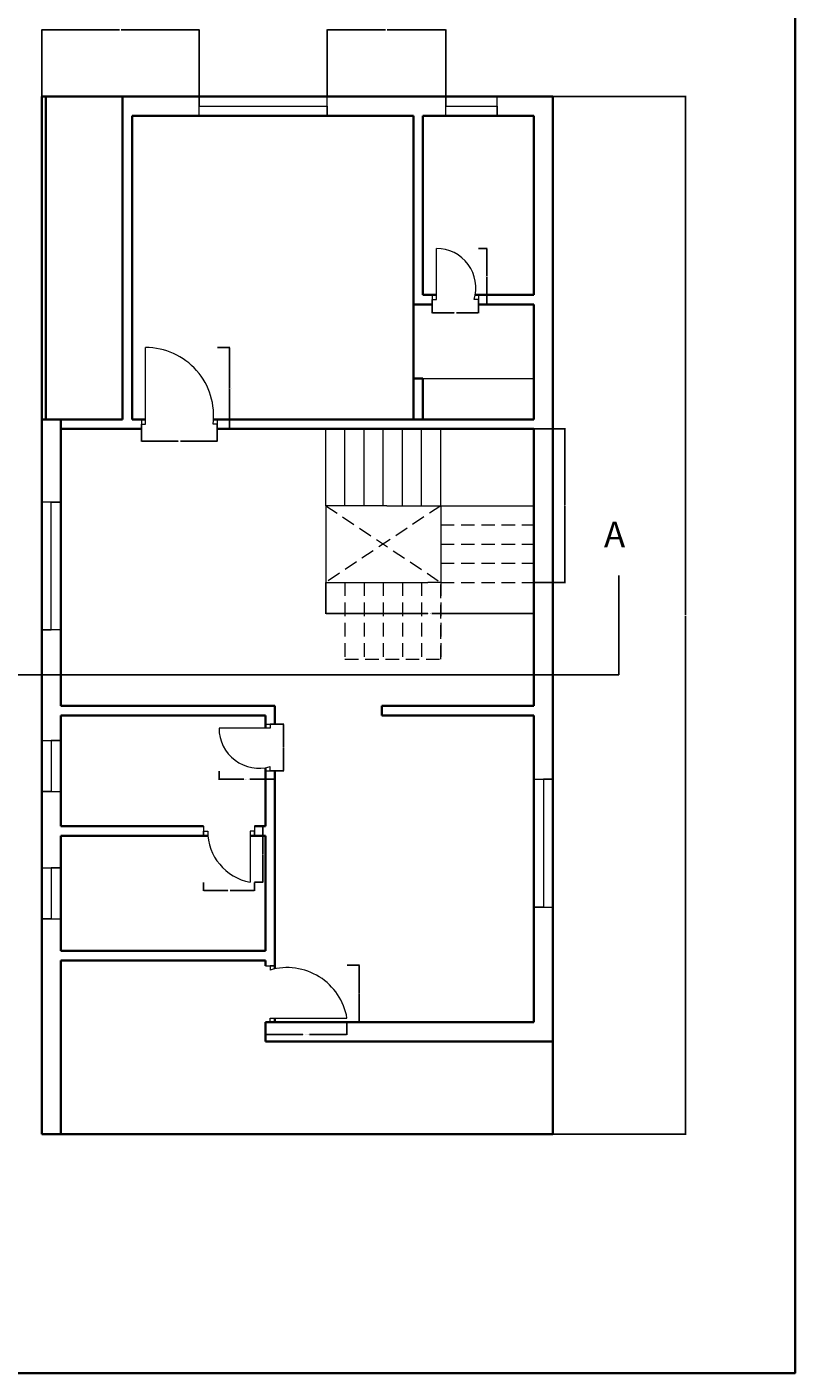
# Model space of a CAD drawing. Units: inches. Extents: x 1911 to 3278, y 2022 to 3108.
# Tile 12 of 13: x 2918 to 3278, y 2022 to 2654. Entities that reach past the tile are written whole.
import ezdxf

# ---------------------------------------------------------------- set-up
doc = ezdxf.new("R2010")
doc.units = ezdxf.units.IN
doc.linetypes.add('DASHED2', pattern=[9.525, 6.35, -3.175])
for name, color, linetype, lineweight in [('A-ANNO-DIMS', 2, 'Continuous', 18), ('A-ANNO-SYMB', 7, 'Continuous', 25), ('A-ANNO-TTLB', 7, 'Continuous', 35), ('A-DOOR', 4, 'Continuous', 18), ('A-FLOR-CASE', 9, 'Continuous', 18), ('A-FLOR-STRS', 7, 'Continuous', 18), ('A-FLOR-STRS-OVHD', 253, 'DASHED2', 13), ('A-GLAZ', 4, 'Continuous', 18), ('A-WALL', 7, 'Continuous', 35)]:
    doc.layers.add(name, color=color, linetype=linetype, lineweight=lineweight)
doc.styles.get("Standard").update_dxf_attribs({"font": 'arial.ttf'})
doc.dimstyles.get("Standard").update_dxf_attribs({"dimtxt": 0.18, "dimasz": 0.18, "dimexe": 0.18, "dimexo": 0.0625, "dimgap": 0.09, "dimtad": 0, "dimtih": 1, "dimtoh": 1, "dimdec": 4, "dimzin": 0, "dimdsep": 46, "dimtxsty": 'Standard', "dimcen": 0.09, "dimadec": 0, "dimazin": 0, "dimtfac": 1, "dimtdec": 4, "dimtofl": 0, "dimtmove": 0, "dimatfit": 3, "dimfxl": 1, "dimtolj": 1, "dimtzin": 0, "dimarcsym": 0})

# ---------------------------------------------------------------- blocks, each defined once
blk = doc.blocks.new('WIN-60')
for p, q in [((0, 60), (9, 60)), ((9, 60), (4.5, 60)), ((4.5, 60), (4.5, 0)), ((4.5, 0), (0, 0)), ((0, 0), (9, 0))]:
    blk.add_line(p, q)
blk = doc.blocks.new('WIN-24')
for p, q in [((0, 24), (9, 24)), ((9, 24), (4.5, 24)), ((4.5, 24), (4.5, 0)), ((4.5, 0), (0, 0)), ((0, 0), (9, 0))]:
    blk.add_line(p, q)
blk = doc.blocks.new('DOOR-BED-FF')
for p, q in [((2, 2.25), (2, 38.25)), ((0, 4.5), (0, 0)), ((0, 0), (0, 2.25)), ((0, 2.25), (2, 2.25)), ((35.66, 2.25), (33.66, 2.25)), ((35.66, 4.5), (35.66, 0)), ((35.66, 0), (35.66, 2.25))]:
    blk.add_line(p, q)
blk.add_arc((2, 6.33), 31.92, 352.65052, 90)
blk = doc.blocks.new('DOOR-BATH-FF')
for p, q in [((2, 2.25), (2, 26.25)), ((0, 4.5), (0, 0)), ((0, 0), (0, 2.25)), ((0, 2.25), (2, 2.25)), ((21.7, 2.25), (19.7, 2.25)), ((21.7, 4.5), (21.7, 0)), ((21.7, 0), (21.7, 2.25))]:
    blk.add_line(p, q)
blk.add_arc((2, 7.72), 18.53, 342.82983, 90)
blk = doc.blocks.new('DOOR-BALCONY')
for p, q in [((0, 26.53), (4.5, 26.53)), ((4.5, 26.53), (2.25, 26.53)), ((2.25, 26.53), (2.25, 24.53)), ((2.32, 0), (2.32, 2)), ((2.32, 2), (38.32, 2))]:
    blk.add_line(p, q)
blk.add_arc((10.23, -2.83), 28.5, 9.76334, 106.26632)
blk = doc.blocks.new('DOOR-DRESS-FF')
for p, q in [((24, 20), (0, 20)), ((21.75, 22), (26.25, 22)), ((26.25, 22), (24, 22)), ((24, 22), (24, 20)), ((21.75, 0), (26.25, 0)), ((24, 0), (24, 2)), ((26.25, 0), (24, 0))]:
    blk.add_line(p, q)
blk.add_arc((18.75, 20), 18.75, 180, 286.25091)
blk = doc.blocks.new('DOOR-ENSUITE-FF')
for p, q in [((0, 26.25), (0, 21.75)), ((23.93, 26.25), (23.93, 21.75)), ((0, 21.75), (0, 24)), ((0, 24), (0, 24)), ((0, 24), (2, 24)), ((23.93, 24), (21.93, 24)), ((21.93, 24), (21.93, 0)), ((23.93, 21.75), (23.93, 24))]:
    blk.add_line(p, q)
blk.add_arc((26.42, 24), 24.42, 180, 259.41225)
blk = doc.blocks.new('STAIR-PLAN-FF')
for p, q in [((0, 36), (0, 72)), ((9, 36), (9, 72)), ((18, 36), (18, 72)), ((27, 36), (27, 72)), ((36, 36), (36, 72)), ((45, 36), (45, 72)), ((54, 36), (54, 72)), ((28.63, 36), (0, 36)), ((0, 36), (0, 0)), ((28.63, 36), (97.65, 36)), ((54, 36), (54, 0)), ((54, 36), (54, 27)), ((0, 0), (48, 0)), ((54, 0), (48, 0))]:
    blk.add_line(p, q)
blk = doc.blocks.new('STAIR-BEYOND-FF')
for p, q in [((54, 72), (0, 36)), ((0, 72), (54, 36)), ((54, 72), (54, 63)), ((54, 63), (97.65, 63)), ((54, 54), (97.65, 54)), ((54, 45), (97.65, 45)), ((9, 36), (9, 0)), ((18, 36), (18, 0)), ((27, 36), (27, 0)), ((36, 36), (36, 0)), ((45, 36), (45, 0)), ((54, 36), (97.65, 36)), ((54, 0), (54, 36)), ((54, 36), (54, 0)), ((9, 0), (54, 0))]:
    blk.add_line(p, q)
blk = doc.blocks.new('*D46')
at = {"layer": 'A-ANNO-DIMS', "color": 0, "lineweight": -2, "transparency": 16777216}
for p, q in [((3007.14, 2503.12), (3012.99, 2503.12)), ((3012.81, 2502.94), (3012.81, 2484.18)), ((3012.81, 2465.05), (3012.81, 2483.82)), ((3007.14, 2464.87), (3012.99, 2464.87))]:
    blk.add_line(p, q, dxfattribs=at)
at = {"layer": 'A-ANNO-DIMS', "color": 0, "transparency": 16777216}
for points in [[(3012.78, 2502.94), (3012.84, 2502.94), (3012.81, 2503.12)], [(3012.78, 2465.05), (3012.84, 2465.05), (3012.81, 2464.87)]]:
    blk.add_solid(points, dxfattribs=at)
at = {"layer": 'Defpoints', "color": 0, "transparency": 16777216}
for p in [(3007.08, 2503.12), (3012.81, 2503.12), (3007.08, 2464.87)]:
    blk.add_point(p, dxfattribs=at)
at = {"layer": 'A-ANNO-DIMS', "color": 0, "transparency": 16777216, "insert": (3012.81, 2484), "char_height": 0.18, "attachment_point": 5}
blk.add_mtext('\\A1;BEDROOM DOOR 38 TYP.', dxfattribs=at)
blk = doc.blocks.new('*D47')
at = {"layer": 'A-ANNO-DIMS', "color": 0, "lineweight": -2, "transparency": 16777216}
for p, q in [((2971.42, 2464.81), (2971.42, 2458.96)), ((3007.08, 2464.81), (3007.08, 2458.96)), ((2971.6, 2459.14), (2988.72, 2459.14)), ((3006.9, 2459.14), (2989.78, 2459.14))]:
    blk.add_line(p, q, dxfattribs=at)
at = {"layer": 'A-ANNO-DIMS', "color": 0, "transparency": 16777216}
for points in [[(2971.6, 2459.17), (2971.6, 2459.11), (2971.42, 2459.14)], [(3006.9, 2459.17), (3006.9, 2459.11), (3007.08, 2459.14)]]:
    blk.add_solid(points, dxfattribs=at)
at = {"layer": 'Defpoints', "color": 0, "transparency": 16777216}
for p in [(2971.42, 2464.87), (3007.08, 2464.87), (3007.08, 2459.14)]:
    blk.add_point(p, dxfattribs=at)
at = {"layer": 'A-ANNO-DIMS', "color": 0, "transparency": 16777216, "insert": (2989.25, 2459.14), "char_height": 0.18, "attachment_point": 5}
blk.add_mtext('\\A1;36 TYP.', dxfattribs=at)
blk = doc.blocks.new('*D48')
at = {"layer": 'A-ANNO-DIMS', "color": 0, "lineweight": -2, "transparency": 16777216}
for p, q in [((3129.7, 2549.62), (3133.76, 2549.62)), ((3133.58, 2549.44), (3133.58, 2536.68)), ((3133.58, 2523.55), (3133.58, 2536.32)), ((3129.7, 2523.37), (3133.76, 2523.37))]:
    blk.add_line(p, q, dxfattribs=at)
at = {"layer": 'A-ANNO-DIMS', "color": 0, "transparency": 16777216}
for points in [[(3133.55, 2549.44), (3133.61, 2549.44), (3133.58, 2549.62)], [(3133.55, 2523.55), (3133.61, 2523.55), (3133.58, 2523.37)]]:
    blk.add_solid(points, dxfattribs=at)
at = {"layer": 'Defpoints', "color": 0, "transparency": 16777216}
for p in [(3129.64, 2549.62), (3133.58, 2549.62), (3129.64, 2523.37)]:
    blk.add_point(p, dxfattribs=at)
at = {"layer": 'A-ANNO-DIMS', "color": 0, "transparency": 16777216, "insert": (3133.58, 2536.5), "char_height": 0.18, "attachment_point": 5}
blk.add_mtext('\\A1;BATH DOOR 26 TYP.', dxfattribs=at)
blk = doc.blocks.new('*D49')
at = {"layer": 'A-ANNO-DIMS', "color": 0, "lineweight": -2, "transparency": 16777216}
for p, q in [((3107.93, 2523.31), (3107.93, 2519.26)), ((3129.64, 2523.31), (3129.64, 2519.26)), ((3108.11, 2519.44), (3118.26, 2519.44)), ((3129.46, 2519.44), (3119.32, 2519.44))]:
    blk.add_line(p, q, dxfattribs=at)
at = {"layer": 'A-ANNO-DIMS', "color": 0, "transparency": 16777216}
for points in [[(3108.11, 2519.47), (3108.11, 2519.41), (3107.93, 2519.44)], [(3129.46, 2519.47), (3129.46, 2519.41), (3129.64, 2519.44)]]:
    blk.add_solid(points, dxfattribs=at)
at = {"layer": 'Defpoints', "color": 0, "transparency": 16777216}
for p in [(3107.93, 2523.37), (3129.64, 2523.37), (3129.64, 2519.44)]:
    blk.add_point(p, dxfattribs=at)
at = {"layer": 'A-ANNO-DIMS', "color": 0, "transparency": 16777216, "insert": (3118.79, 2519.44), "char_height": 0.18, "attachment_point": 5}
blk.add_mtext('\\A1;22 TYP.', dxfattribs=at)
blk = doc.blocks.new('*D50')
at = {"layer": 'A-ANNO-DIMS', "color": 0, "lineweight": -2, "transparency": 16777216}
for p, q in [((3029.64, 2186.31), (3029.64, 2180.45)), ((3067.96, 2186.31), (3067.96, 2180.45)), ((3029.82, 2180.63), (3047.23, 2180.63)), ((3067.78, 2180.63), (3050.37, 2180.63))]:
    blk.add_line(p, q, dxfattribs=at)
at = {"layer": 'A-ANNO-DIMS', "color": 0, "transparency": 16777216}
for points in [[(3029.82, 2180.66), (3029.82, 2180.6), (3029.64, 2180.63)], [(3067.78, 2180.66), (3067.78, 2180.6), (3067.96, 2180.63)]]:
    blk.add_solid(points, dxfattribs=at)
at = {"layer": 'Defpoints', "color": 0, "transparency": 16777216}
for p in [(3029.64, 2186.37), (3067.96, 2186.37), (3067.96, 2180.63)]:
    blk.add_point(p, dxfattribs=at)
at = {"layer": 'A-ANNO-DIMS', "color": 0, "transparency": 16777216, "insert": (3048.8, 2180.63), "char_height": 0.18, "attachment_point": 5}
blk.add_mtext('\\A1;BALCONY DOOR 38 TYP.', dxfattribs=at)
blk = doc.blocks.new('*D51')
at = {"layer": 'A-ANNO-DIMS', "color": 0, "lineweight": -2, "transparency": 16777216}
for p, q in [((3068.02, 2213.17), (3073.89, 2213.17)), ((3073.71, 2212.99), (3073.71, 2199.95)), ((3073.71, 2186.55), (3073.71, 2199.59)), ((3068.02, 2186.37), (3073.89, 2186.37))]:
    blk.add_line(p, q, dxfattribs=at)
at = {"layer": 'A-ANNO-DIMS', "color": 0, "transparency": 16777216}
for points in [[(3073.68, 2212.99), (3073.74, 2212.99), (3073.71, 2213.17)], [(3073.68, 2186.55), (3073.74, 2186.55), (3073.71, 2186.37)]]:
    blk.add_solid(points, dxfattribs=at)
at = {"layer": 'Defpoints', "color": 0, "transparency": 16777216}
for p in [(3067.96, 2213.17), (3073.71, 2213.17), (3067.96, 2186.37)]:
    blk.add_point(p, dxfattribs=at)
at = {"layer": 'A-ANNO-DIMS', "color": 0, "transparency": 16777216, "insert": (3073.71, 2199.77), "char_height": 0.18, "attachment_point": 5}
blk.add_mtext('\\A1;27 TYP.', dxfattribs=at)
blk = doc.blocks.new('*D52')
at = {"layer": 'A-ANNO-DIMS', "color": 0, "lineweight": -2, "transparency": 16777216}
for p, q in [((3007.89, 2304.31), (3007.89, 2300.26)), ((3008.07, 2300.44), (3019.61, 2300.44)), ((3033.96, 2300.44), (3022.42, 2300.44)), ((3034.14, 2304.31), (3034.14, 2300.26))]:
    blk.add_line(p, q, dxfattribs=at)
at = {"layer": 'A-ANNO-DIMS', "color": 0, "transparency": 16777216}
for points in [[(3008.07, 2300.47), (3008.07, 2300.41), (3007.89, 2300.44)], [(3033.96, 2300.47), (3033.96, 2300.41), (3034.14, 2300.44)]]:
    blk.add_solid(points, dxfattribs=at)
at = {"layer": 'Defpoints', "color": 0, "transparency": 16777216}
for p in [(3007.89, 2304.37), (3034.14, 2304.37), (3034.14, 2300.44)]:
    blk.add_point(p, dxfattribs=at)
at = {"layer": 'A-ANNO-DIMS', "color": 0, "transparency": 16777216, "insert": (3021.01, 2300.44), "char_height": 0.18, "attachment_point": 5}
blk.add_mtext('\\A1;DRESS DOOR 26 TYP.', dxfattribs=at)
blk = doc.blocks.new('*D53')
at = {"layer": 'A-ANNO-DIMS', "color": 0, "lineweight": -2, "transparency": 16777216}
for p, q in [((3034.2, 2326.38), (3038.26, 2326.38)), ((3038.08, 2326.2), (3038.08, 2315.56)), ((3038.08, 2304.55), (3038.08, 2315.19)), ((3034.2, 2304.37), (3038.26, 2304.37))]:
    blk.add_line(p, q, dxfattribs=at)
at = {"layer": 'A-ANNO-DIMS', "color": 0, "transparency": 16777216}
for points in [[(3038.05, 2326.2), (3038.11, 2326.2), (3038.08, 2326.38)], [(3038.05, 2304.55), (3038.11, 2304.55), (3038.08, 2304.37)]]:
    blk.add_solid(points, dxfattribs=at)
at = {"layer": 'Defpoints', "color": 0, "transparency": 16777216}
for p in [(3034.14, 2326.38), (3038.08, 2326.38), (3034.14, 2304.37)]:
    blk.add_point(p, dxfattribs=at)
at = {"layer": 'A-ANNO-DIMS', "color": 0, "transparency": 16777216, "insert": (3038.08, 2315.37), "char_height": 0.18, "attachment_point": 5}
blk.add_mtext('\\A1;22 TYP.', dxfattribs=at)
blk = doc.blocks.new('*D54')
at = {"layer": 'A-ANNO-DIMS', "color": 0, "lineweight": -2, "transparency": 16777216}
for p, q in [((3024.55, 2278.37), (3028.61, 2278.37)), ((3028.43, 2278.19), (3028.43, 2265.43)), ((3028.43, 2252.3), (3028.43, 2265.07)), ((3024.55, 2252.12), (3028.61, 2252.12))]:
    blk.add_line(p, q, dxfattribs=at)
at = {"layer": 'A-ANNO-DIMS', "color": 0, "transparency": 16777216}
for points in [[(3028.4, 2278.19), (3028.46, 2278.19), (3028.43, 2278.37)], [(3028.4, 2252.3), (3028.46, 2252.3), (3028.43, 2252.12)]]:
    blk.add_solid(points, dxfattribs=at)
at = {"layer": 'Defpoints', "color": 0, "transparency": 16777216}
for p in [(3024.49, 2278.37), (3028.43, 2278.37), (3024.49, 2252.12)]:
    blk.add_point(p, dxfattribs=at)
at = {"layer": 'A-ANNO-DIMS', "color": 0, "transparency": 16777216, "insert": (3028.43, 2265.25), "char_height": 0.18, "attachment_point": 5}
blk.add_mtext('\\A1;ENSUITE DOOR 26 TYP.', dxfattribs=at)
blk = doc.blocks.new('*D55')
at = {"layer": 'A-ANNO-DIMS', "color": 0, "lineweight": -2, "transparency": 16777216}
for p, q in [((3000.56, 2252.06), (3000.56, 2248.01)), ((3024.49, 2252.06), (3024.49, 2248.01)), ((3000.74, 2248.19), (3011.99, 2248.19)), ((3024.31, 2248.19), (3013.05, 2248.19))]:
    blk.add_line(p, q, dxfattribs=at)
at = {"layer": 'A-ANNO-DIMS', "color": 0, "transparency": 16777216}
for points in [[(3000.74, 2248.22), (3000.74, 2248.16), (3000.56, 2248.19)], [(3024.31, 2248.22), (3024.31, 2248.16), (3024.49, 2248.19)]]:
    blk.add_solid(points, dxfattribs=at)
at = {"layer": 'Defpoints', "color": 0, "transparency": 16777216}
for p in [(3000.56, 2252.12), (3024.49, 2252.12), (3024.49, 2248.19)]:
    blk.add_point(p, dxfattribs=at)
at = {"layer": 'A-ANNO-DIMS', "color": 0, "transparency": 16777216, "insert": (3012.52, 2248.19), "char_height": 0.18, "attachment_point": 5}
blk.add_mtext('\\A1;24 TYP.', dxfattribs=at)
blk = doc.blocks.new('*D62')
at = {"layer": 'A-ANNO-DIMS', "color": 0, "lineweight": -2, "transparency": 16777216}
for p, q in [((3057.99, 2392.81), (3057.99, 2378.05)), ((3155.64, 2392.81), (3155.64, 2378.05)), ((3058.17, 2378.23), (3105.88, 2378.23)), ((3155.46, 2378.23), (3107.75, 2378.23))]:
    blk.add_line(p, q, dxfattribs=at)
at = {"layer": 'A-ANNO-DIMS', "color": 0, "transparency": 16777216}
for points in [[(3058.17, 2378.26), (3058.17, 2378.2), (3057.99, 2378.23)], [(3155.46, 2378.26), (3155.46, 2378.2), (3155.64, 2378.23)]]:
    blk.add_solid(points, dxfattribs=at)
at = {"layer": 'Defpoints', "color": 0, "transparency": 16777216}
for p in [(3057.99, 2392.87), (3155.64, 2392.87), (3155.64, 2378.23)]:
    blk.add_point(p, dxfattribs=at)
at = {"layer": 'A-ANNO-DIMS', "color": 0, "transparency": 16777216, "insert": (3106.81, 2378.23), "char_height": 0.18, "attachment_point": 5}
blk.add_mtext('\\A1;STAIR 98 TYP.', dxfattribs=at)
blk = doc.blocks.new('*D63')
at = {"layer": 'A-ANNO-DIMS', "color": 0, "lineweight": -2, "transparency": 16777216}
for p, q in [((3155.7, 2464.87), (3170.47, 2464.87)), ((3170.29, 2464.69), (3170.29, 2429.05)), ((3170.29, 2393.05), (3170.29, 2428.69)), ((3155.7, 2392.87), (3170.47, 2392.87))]:
    blk.add_line(p, q, dxfattribs=at)
at = {"layer": 'A-ANNO-DIMS', "color": 0, "transparency": 16777216}
for points in [[(3170.26, 2464.69), (3170.32, 2464.69), (3170.29, 2464.87)], [(3170.26, 2393.05), (3170.32, 2393.05), (3170.29, 2392.87)]]:
    blk.add_solid(points, dxfattribs=at)
at = {"layer": 'Defpoints', "color": 0, "transparency": 16777216}
for p in [(3155.64, 2464.87), (3170.29, 2464.87), (3155.64, 2392.87)]:
    blk.add_point(p, dxfattribs=at)
at = {"layer": 'A-ANNO-DIMS', "color": 0, "transparency": 16777216, "insert": (3170.29, 2428.87), "char_height": 0.18, "attachment_point": 5}
blk.add_mtext('\\A1;72 TYP.', dxfattribs=at)
blk = doc.blocks.new('*D84')
at = {"layer": 'A-ANNO-DIMS', "color": 0, "lineweight": -2, "transparency": 16777216}
for p, q in [((2924.64, 2620.94), (2924.64, 2652.45)), ((2924.82, 2652.27), (2961.22, 2652.27)), ((2998.41, 2652.27), (2962.01, 2652.27)), ((2998.59, 2620.94), (2998.59, 2652.45))]:
    blk.add_line(p, q, dxfattribs=at)
at = {"layer": 'A-ANNO-DIMS', "color": 0, "transparency": 16777216}
for points in [[(2924.82, 2652.3), (2924.82, 2652.24), (2924.64, 2652.27)], [(2998.41, 2652.3), (2998.41, 2652.24), (2998.59, 2652.27)]]:
    blk.add_solid(points, dxfattribs=at)
at = {"layer": 'Defpoints', "color": 0, "transparency": 16777216}
for p in [(2998.59, 2652.27), (2924.64, 2620.87), (2998.59, 2620.87)]:
    blk.add_point(p, dxfattribs=at)
at = {"layer": 'A-ANNO-DIMS', "color": 0, "transparency": 16777216, "insert": (2961.61, 2652.27), "char_height": 0.18, "attachment_point": 5}
blk.add_mtext('\\A1;73.95', dxfattribs=at)
blk = doc.blocks.new('*D85')
at = {"layer": 'A-ANNO-DIMS', "color": 0, "lineweight": -2, "transparency": 16777216}
for p, q in [((3058.59, 2620.94), (3058.59, 2652.45)), ((3058.77, 2652.27), (3086.11, 2652.27)), ((3114.23, 2652.27), (3086.89, 2652.27)), ((3114.41, 2620.94), (3114.41, 2652.45))]:
    blk.add_line(p, q, dxfattribs=at)
at = {"layer": 'A-ANNO-DIMS', "color": 0, "transparency": 16777216}
for points in [[(3058.77, 2652.3), (3058.77, 2652.24), (3058.59, 2652.27)], [(3114.23, 2652.3), (3114.23, 2652.24), (3114.41, 2652.27)]]:
    blk.add_solid(points, dxfattribs=at)
at = {"layer": 'Defpoints', "color": 0, "transparency": 16777216}
for p in [(3114.41, 2652.27), (3058.59, 2620.87), (3114.41, 2620.87)]:
    blk.add_point(p, dxfattribs=at)
at = {"layer": 'A-ANNO-DIMS', "color": 0, "transparency": 16777216, "insert": (3086.5, 2652.27), "char_height": 0.18, "attachment_point": 5}
blk.add_mtext('\\A1;55.83', dxfattribs=at)
blk = doc.blocks.new('*D86')
at = {"layer": 'A-ANNO-DIMS', "color": 0, "lineweight": -2, "transparency": 16777216}
for p, q in [((3164.7, 2620.87), (3227.12, 2620.87)), ((3226.94, 2620.69), (3226.94, 2377.56)), ((3226.94, 2134.05), (3226.94, 2377.19)), ((3164.7, 2133.87), (3227.12, 2133.87))]:
    blk.add_line(p, q, dxfattribs=at)
at = {"layer": 'A-ANNO-DIMS', "color": 0, "transparency": 16777216}
for points in [[(3226.91, 2620.69), (3226.97, 2620.69), (3226.94, 2620.87)], [(3226.91, 2134.05), (3226.97, 2134.05), (3226.94, 2133.87)]]:
    blk.add_solid(points, dxfattribs=at)
at = {"layer": 'Defpoints', "color": 0, "transparency": 16777216}
for p in [(3164.64, 2620.87), (3226.94, 2620.87), (3164.64, 2133.87)]:
    blk.add_point(p, dxfattribs=at)
at = {"layer": 'A-ANNO-DIMS', "color": 0, "transparency": 16777216, "insert": (3226.94, 2377.37), "char_height": 0.18, "attachment_point": 5}
blk.add_mtext('\\A1;487', dxfattribs=at)

msp = doc.modelspace()

# ---------------------------------------------------------------- linework, layer by layer
at = {"layer": 'A-ANNO-SYMB'}
for q in [(3195.5436, 2396.0454), (2593.3449, 2349.5267)]:
    msp.add_line((3195.5436, 2349.5267), q, dxfattribs=at)
at = {"layer": 'A-ANNO-TTLB'}
msp.add_lwpolyline([(1911.3875, 3108.0628), (3278.3142, 3108.0628), (3278.3142, 2021.7237), (1911.3875, 2021.7237)], close=True, dxfattribs=at)
at = {"layer": 'A-FLOR-CASE'}
msp.add_line((3099.1387, 2488.532), (3155.6387, 2488.532), dxfattribs=at)
at = {"layer": 'A-WALL'}
for p, q in [((2924.6387, 2620.8733), (3164.6387, 2620.8733)), ((2924.6387, 2620.8733), (2924.6387, 2133.8733)), ((2926.6387, 2473.8733), (2926.6387, 2620.8733)), ((2962.6387, 2611.8733), (2962.6387, 2620.8733)), ((3164.6387, 2620.8733), (3164.6387, 2133.8733)), ((2962.6387, 2611.8733), (2962.6387, 2469.3733)), ((2967.1387, 2611.8733), (3099.1387, 2611.8733)), ((2967.1387, 2611.8733), (2967.1387, 2469.3733)), ((3099.1387, 2611.8733), (3099.1387, 2469.3733)), ((3103.6387, 2611.8733), (3155.6387, 2611.8733)), ((3103.6387, 2611.8733), (3103.6387, 2527.8733)), ((3155.6387, 2611.8733), (3155.6387, 2527.8733)), ((3103.6387, 2527.8733), (3109.9348, 2527.8733)), ((3128.1826, 2527.8733), (3155.6387, 2527.8733)), ((3103.6387, 2523.3733), (3099.1387, 2523.3733)), ((3103.6387, 2523.3733), (3107.9348, 2523.3733)), ((3129.6387, 2523.3733), (3155.6387, 2523.3733)), ((3155.6387, 2523.3733), (3155.6387, 2469.3733)), ((3103.6387, 2488.532), (3099.1387, 2488.532)), ((3103.6387, 2488.532), (3103.6387, 2469.3733)), ((2926.6387, 2469.3733), (2926.6387, 2473.8733)), ((2933.6387, 2469.3733), (2924.6387, 2469.3733)), ((2924.6387, 2469.3733), (2926.6387, 2469.3733)), ((2933.6387, 2469.3733), (2962.6387, 2469.3733)), ((2933.6387, 2469.3733), (2933.6387, 2334.8733)), ((2933.6387, 2464.8733), (2971.421, 2464.8733)), ((2967.1387, 2469.3733), (2973.421, 2469.3733)), ((3005.2854, 2469.3733), (3155.6387, 2469.3733)), ((3007.0759, 2464.8733), (3155.6387, 2464.8733)), ((3155.6387, 2464.8733), (3155.6387, 2334.8733)), ((2933.6387, 2334.8733), (3034.1387, 2334.8733)), ((3034.1387, 2330.3733), (3034.1387, 2334.8733)), ((3084.2941, 2330.3733), (3084.2941, 2334.8733)), ((3084.2941, 2334.8733), (3155.6387, 2334.8733)), ((2933.6387, 2330.3733), (3029.6387, 2330.3733)), ((2933.6387, 2330.3733), (2933.6387, 2278.3733)), ((3029.6387, 2330.3733), (3029.6387, 2324.3763)), ((3034.1387, 2330.3733), (3034.1387, 2326.3763)), ((3084.2941, 2330.3733), (3155.6387, 2330.3733)), ((3155.6387, 2330.3733), (3155.6387, 2186.3733)), ((3029.6387, 2305.8652), (3029.6387, 2278.3733)), ((3034.1387, 2304.3733), (3034.1387, 2215.3733)), ((2933.6387, 2278.3733), (3000.5586, 2278.3733)), ((3024.4881, 2278.3733), (3029.6387, 2278.3733)), ((2933.6387, 2273.8733), (3002.6625, 2273.8733)), ((2933.6387, 2273.8733), (2933.6387, 2219.8733)), ((3022.4881, 2273.8733), (3029.6387, 2273.8733)), ((3029.6387, 2273.8733), (3029.6387, 2219.8733)), ((2933.6387, 2219.8733), (3029.6387, 2219.8733)), ((2933.6387, 2215.3733), (3029.6387, 2215.3733)), ((2933.6387, 2215.3733), (2933.6387, 2133.8733)), ((3029.6387, 2215.3733), (3029.6387, 2212.8991)), ((3034.1387, 2215.3733), (3034.1387, 2211.4574)), ((3029.6387, 2186.3733), (3155.6387, 2186.3733)), ((3029.6387, 2186.3733), (3029.6387, 2177.3733)), ((3034.1387, 2188.3733), (3034.1387, 2186.3733)), ((3029.6387, 2177.3733), (3155.6387, 2177.3733)), ((3155.6387, 2177.3733), (3164.6387, 2177.3733)), ((2924.6387, 2133.8733), (3164.6387, 2133.8733))]:
    msp.add_line(p, q, dxfattribs=at)

# ---------------------------------------------------------------- block references
at = {"layer": 'A-DOOR'}
for name, p in [('DOOR-BATH-FF', (3107.9345, 2523.373)), ('DOOR-BED-FF', (2971.4205, 2464.873)), ('DOOR-DRESS-FF', (3007.8885, 2304.373)), ('DOOR-ENSUITE-FF', (3000.5585, 2252.123)), ('DOOR-BALCONY', (3029.6385, 2186.373))]:
    msp.add_blockref(name, p, dxfattribs=at)
at = {"layer": 'A-FLOR-STRS'}
msp.add_blockref('STAIR-PLAN-FF', (3057.9895, 2392.873), dxfattribs=at)
at = {"layer": 'A-FLOR-STRS-OVHD'}
msp.add_blockref('STAIR-BEYOND-FF', (3057.9895, 2356.873), dxfattribs=at)
at = {"layer": 'A-GLAZ'}
for name, p, rotation in [('WIN-60', (3058.586, 2611.8729), 90.00000000000286), ('WIN-24', (3138.4124, 2611.8729), 90.00000000000666), ('WIN-60', (2933.6391, 2430.5886), 180)]:
    msp.add_blockref(name, p, dxfattribs=dict(at, rotation=rotation))
for name, p in [('WIN-24', (2924.6383, 2294.6461)), ('WIN-60', (3155.6383, 2240.4658)), ('WIN-24', (2924.6383, 2234.9197))]:
    msp.add_blockref(name, p, dxfattribs=at)

# ---------------------------------------------------------------- texts
at = {"layer": 'A-ANNO-SYMB', "insert": (3188.6021, 2421.345), "char_height": 12, "attachment_point": 1}
msp.add_mtext_dynamic_manual_height_columns('A', width=19.648481, gutter_width=12.5, heights=[0], dxfattribs=at)

# ---------------------------------------------------------------- dimensions: what is measured, and where the dimension line sits
at = {"layer": 'A-ANNO-DIMS'}
for base, p1, p2, picture, middle in [((2998.5857, 2652.2733), (2924.6387, 2620.8733), (2998.5857, 2620.8733), '*D84', (2961.6122, 2652.2733)), ((3114.4122, 2652.2733), (3058.5857, 2620.8733), (3114.4122, 2620.8733), '*D85', (3086.499, 2652.2733))]:
    dim = msp.add_linear_dim(base=base, p1=p1, p2=p2, dimstyle='Standard', override={"dimdec": 2, "dimlfac": 1, "dimrnd": 0, "dimzin": 0, "dimdsep": 46, "dimlunit": 2}, dxfattribs=at)
    dim.commit()
    dim.dimension.update_dxf_attribs({"geometry": picture, "text_midpoint": middle})
dim = msp.add_linear_dim(base=(3226.9436, 2620.8733), p1=(3164.6387, 2133.8733), p2=(3164.6387, 2620.8733), angle=90, dimstyle='Standard', override={"dimdec": 0, "dimlfac": 1, "dimrnd": 0, "dimzin": 0, "dimdsep": 46, "dimlunit": 2}, dxfattribs=at)
dim.commit()
dim.dimension.update_dxf_attribs({"geometry": '*D86', "text_midpoint": (3226.9436, 2377.3733)})
for base, p1, p2, text, picture, middle in [((3133.5762, 2549.6233), (3129.6387, 2523.3733), (3129.6387, 2549.6233), 'BATH DOOR <> TYP.', '*D48', (3133.5762, 2536.4983)), ((3012.8134, 2503.1233), (3007.0759, 2464.8733), (3007.0759, 2503.1233), 'BEDROOM DOOR <> TYP.', '*D46', (3012.8134, 2483.9983)), ((3170.2861, 2464.8733), (3155.6387, 2392.8733), (3155.6387, 2464.8733), '<> TYP.', '*D63', (3170.2861, 2428.8733)), ((3038.0762, 2326.3763), (3034.1387, 2304.3733), (3034.1387, 2326.3763), '<> TYP.', '*D53', (3038.0762, 2315.3748)), ((3028.4256, 2278.3733), (3024.4881, 2252.1233), (3024.4881, 2278.3733), 'ENSUITE DOOR <> TYP.', '*D54', (3028.4256, 2265.2483)), ((3073.7063, 2213.1738), (3067.9584, 2186.3733), (3067.9584, 2213.1738), '<> TYP.', '*D51', (3073.7063, 2199.7735))]:
    dim = msp.add_linear_dim(base=base, p1=p1, p2=p2, angle=90, text=text, dimstyle='Standard', override={"dimdec": 0, "dimlfac": 1, "dimrnd": 0, "dimzin": 0, "dimdsep": 46, "dimlunit": 2}, dxfattribs=at)
    dim.commit()
    dim.dimension.update_dxf_attribs({"geometry": picture, "text_midpoint": middle})
for base, p1, p2, text, picture, middle in [((3129.6387, 2519.4358), (3107.9348, 2523.3733), (3129.6387, 2523.3733), '<> TYP.', '*D49', (3118.7867, 2519.4358)), ((3007.0759, 2459.1358), (2971.421, 2464.8733), (3007.0759, 2464.8733), '<> TYP.', '*D47', (2989.2484, 2459.1358)), ((3155.6387, 2378.2259), (3057.9894, 2392.8733), (3155.6387, 2392.8733), 'STAIR <> TYP.', '*D62', (3106.8141, 2378.2259)), ((3034.1387, 2300.4358), (3007.8887, 2304.3733), (3034.1387, 2304.3733), 'DRESS DOOR <> TYP.', '*D52', (3021.0137, 2300.4358)), ((3024.4881, 2248.1858), (3000.5586, 2252.1233), (3024.4881, 2252.1233), '<> TYP.', '*D55', (3012.5233, 2248.1858)), ((3067.9584, 2180.6253), (3029.6387, 2186.3733), (3067.9584, 2186.3733), 'BALCONY DOOR <> TYP.', '*D50', (3048.7986, 2180.6253))]:
    dim = msp.add_linear_dim(base=base, p1=p1, p2=p2, text=text, dimstyle='Standard', override={"dimdec": 0, "dimlfac": 1, "dimrnd": 0, "dimzin": 0, "dimdsep": 46, "dimlunit": 2}, dxfattribs=at)
    dim.commit()
    dim.dimension.update_dxf_attribs({"geometry": picture, "text_midpoint": middle})

doc.saveas('drawing.dxf')
